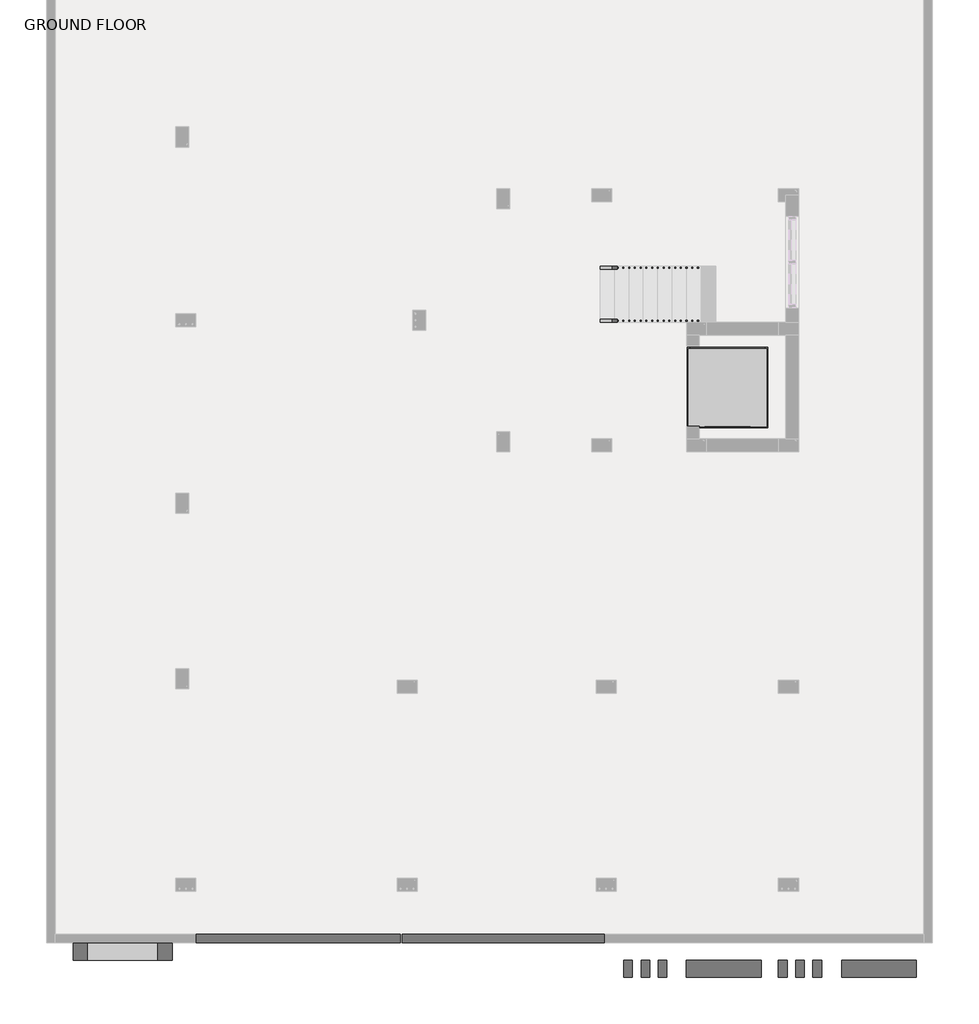
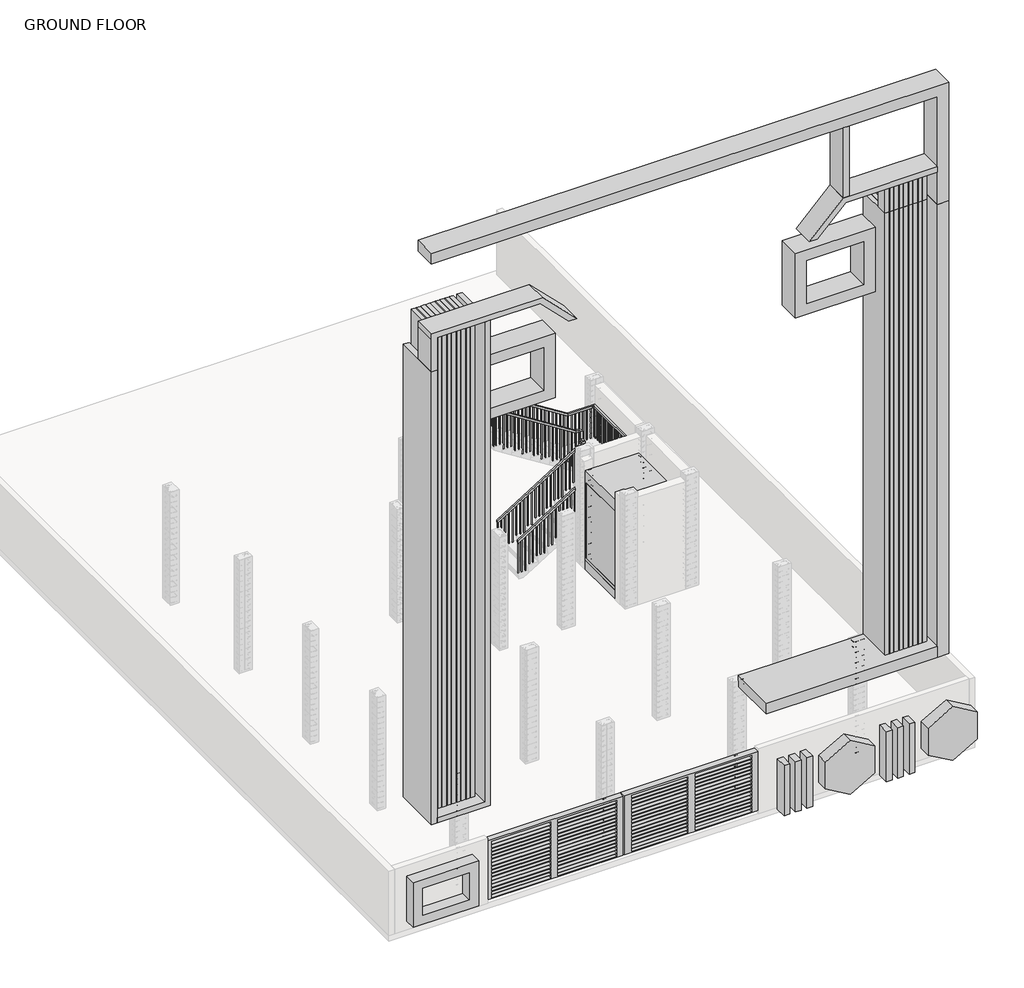
# One storey, part 2 of 7: 2 proxies, 2 railings.
"""IFC4 building model written with IfcOpenShell, lengths in millimetres."""

from ifc_helpers import new_model, si_unit, frame, origin, place, context, project, spatial, polyline, outline, extrude, faceted_brep, transform, mapped, element, save
from components import generic_models_4_generic_models_1_75103227, lift_glass_2_lift_with_hydraulic_ram_a28bd677

model = new_model("IFC4")

# Units and contexts
model_context = context("Model", 3, world=origin())
ifc_project = project(units=[si_unit("LENGTHUNIT", "METRE", prefix="MILLI")], contexts=[model_context])

# Site, building, storey
site = spatial("IfcSite", under=ifc_project)
building = spatial("IfcBuilding", under=site)
storey = spatial("IfcBuildingStorey", under=building, Name="GROUND FLOOR", Elevation=0.0)

# Proxies
placement = place(None, origin())
generic_models_4_generic_models_1_shape = generic_models_4_generic_models_1_75103227(model_context)
element("IfcBuildingElementProxy", 1, Name="Generic Models 4 : Generic Models 1", ObjectType="Generic Models 4 : Generic Models 1", at=placement, inside=storey, context=model_context, shape_type="MappedRepresentation", body=[
    mapped(generic_models_4_generic_models_1_shape, transform((0.0, 0.0, 0.0), x_axis=(1.0, 0.0, 0.0), y_axis=(0.0, 1.0, 0.0), z_axis=(0.0, 0.0, 1.0))),
])
lift_glass_2_lift_with_hydraulic_ram_shape = lift_glass_2_lift_with_hydraulic_ram_a28bd677(model_context)
element("IfcBuildingElementProxy", 2, Name="Lift Glass (2) : Lift with Hydraulic Ram", ObjectType="Lift Glass (2) : Lift with Hydraulic Ram", at=placement, inside=storey, context=model_context, shape_type="MappedRepresentation", body=[
    mapped(lift_glass_2_lift_with_hydraulic_ram_shape, transform((3468.4307677, -1196.2226692, 252.7510845), x_axis=(1.0, 0.0, 0.0), y_axis=(0.0, 1.0, 0.0), z_axis=(0.0, 0.0, 1.0))),
])

# Railings
element("IfcRailing", 3, ObjectType="Handrail - Rectangular", at=placement, inside=storey, context=model_context, shape_type="SolidModel", body=[
    faceted_brep([(1253.5166213, 60.259934, 1074.42), (1253.5166213, 60.259934, 1014.3792137), (1253.5166213, 9.459934, 1014.3792137), (1253.5166213, 9.459934, 1074.42), (3539.5166213, 60.259934, 2514.6), (3554.184536, 60.259934, 2463.8), (3554.184536, 9.459934, 2463.8), (3539.5166213, 9.459934, 2514.6), (4479.3166213, 60.259934, 2514.6), (4479.3166213, 60.259934, 2463.8), (4530.1166213, 9.459934, 2463.8), (4530.1166213, 9.459934, 2514.6), (4479.3166213, 2092.259934, 2514.6), (4479.3166213, 2092.259934, 2463.8), (4530.1166213, 2143.059934, 2463.8), (4530.1166213, 2143.059934, 2514.6), (3793.5166213, 2092.259934, 2514.6), (3778.8487066, 2092.259934, 2463.8), (3778.8487066, 2143.059934, 2463.8), (3793.5166213, 2143.059934, 2514.6), (1253.5166213, 2092.259934, 4114.8), (1253.5166213, 2143.059934, 4114.8), (1253.5166213, 2143.059934, 4054.7592137), (1253.5166213, 2092.259934, 4054.7592137)], [[[0, 1, 2, 3]], [[1, 0, 4, 5]], [[2, 1, 5, 6]], [[3, 2, 6, 7]], [[0, 3, 7, 4]], [[5, 4, 8, 9]], [[6, 5, 9, 10]], [[7, 6, 10, 11]], [[4, 7, 11, 8]], [[9, 8, 12, 13]], [[10, 9, 13, 14]], [[11, 10, 14, 15]], [[8, 11, 15, 12]], [[13, 12, 16, 17]], [[14, 13, 17, 18]], [[15, 14, 18, 19]], [[12, 15, 19, 16]], [[20, 21, 22, 23]], [[17, 16, 20, 23]], [[18, 17, 23, 22]], [[19, 18, 22, 21]], [[16, 19, 21, 20]]]),
    extrude(outline(polyline([(3984.7504637, 1364.6416213), (3996.7519637, 1345.5916213), (3040.38, 1345.5916213), (3040.38, 1364.6416213), (3984.7504637, 1364.6416213)])), frame((0.0, 2108.134934, 0.0), z_axis=(0.0, 1.0, 0.0), x_axis=(0.0, 0.0, 1.0)), (0.0, 0.0, 1.0), 19.05),
    extrude(outline(polyline([(3920.7424637, 1466.2416213), (3932.7439637, 1447.1916213), (3040.38, 1447.1916213), (3040.38, 1466.2416213), (3920.7424637, 1466.2416213)])), frame((0.0, 2108.134934, 0.0), z_axis=(0.0, 1.0, 0.0), x_axis=(0.0, 0.0, 1.0)), (0.0, 0.0, 1.0), 19.05),
    extrude(outline(polyline([(3856.7344637, 1567.8416213), (3868.7359637, 1548.7916213), (2880.36, 1548.7916213), (2880.36, 1567.8416213), (3856.7344637, 1567.8416213)])), frame((0.0, 2108.134934, 0.0), z_axis=(0.0, 1.0, 0.0), x_axis=(0.0, 0.0, 1.0)), (0.0, 0.0, 1.0), 19.05),
    extrude(outline(polyline([(3792.7264637, 1669.4416213), (3804.7279637, 1650.3916213), (2880.36, 1650.3916213), (2880.36, 1669.4416213), (3792.7264637, 1669.4416213)])), frame((0.0, 2108.134934, 0.0), z_axis=(0.0, 1.0, 0.0), x_axis=(0.0, 0.0, 1.0)), (0.0, 0.0, 1.0), 19.05),
    extrude(outline(polyline([(3728.7184637, 1771.0416213), (3740.7199637, 1751.9916213), (2880.36, 1751.9916213), (2880.36, 1771.0416213), (3728.7184637, 1771.0416213)])), frame((0.0, 2108.134934, 0.0), z_axis=(0.0, 1.0, 0.0), x_axis=(0.0, 0.0, 1.0)), (0.0, 0.0, 1.0), 19.05),
    extrude(outline(polyline([(3664.7104637, 1872.6416213), (3676.7119637, 1853.5916213), (2720.34, 1853.5916213), (2720.34, 1872.6416213), (3664.7104637, 1872.6416213)])), frame((0.0, 2108.134934, 0.0), z_axis=(0.0, 1.0, 0.0), x_axis=(0.0, 0.0, 1.0)), (0.0, 0.0, 1.0), 19.05),
    extrude(outline(polyline([(3600.7024637, 1974.2416213), (3612.7039637, 1955.1916213), (2720.34, 1955.1916213), (2720.34, 1974.2416213), (3600.7024637, 1974.2416213)])), frame((0.0, 2108.134934, 0.0), z_axis=(0.0, 1.0, 0.0), x_axis=(0.0, 0.0, 1.0)), (0.0, 0.0, 1.0), 19.05),
    extrude(outline(polyline([(3536.6944637, 2075.8416213), (3548.6959637, 2056.7916213), (2560.32, 2056.7916213), (2560.32, 2075.8416213), (3536.6944637, 2075.8416213)])), frame((0.0, 2108.134934, 0.0), z_axis=(0.0, 1.0, 0.0), x_axis=(0.0, 0.0, 1.0)), (0.0, 0.0, 1.0), 19.05),
    extrude(outline(polyline([(3472.6864637, 2177.4416213), (3484.6879637, 2158.3916213), (2560.32, 2158.3916213), (2560.32, 2177.4416213), (3472.6864637, 2177.4416213)])), frame((0.0, 2108.134934, 0.0), z_axis=(0.0, 1.0, 0.0), x_axis=(0.0, 0.0, 1.0)), (0.0, 0.0, 1.0), 19.05),
    extrude(outline(polyline([(3408.6784637, 2279.0416213), (3420.6799637, 2259.9916213), (2560.32, 2259.9916213), (2560.32, 2279.0416213), (3408.6784637, 2279.0416213)])), frame((0.0, 2108.134934, 0.0), z_axis=(0.0, 1.0, 0.0), x_axis=(0.0, 0.0, 1.0)), (0.0, 0.0, 1.0), 19.05),
    extrude(outline(polyline([(3344.6704637, 2380.6416213), (3356.6719637, 2361.5916213), (2400.3, 2361.5916213), (2400.3, 2380.6416213), (3344.6704637, 2380.6416213)])), frame((0.0, 2108.134934, 0.0), z_axis=(0.0, 1.0, 0.0), x_axis=(0.0, 0.0, 1.0)), (0.0, 0.0, 1.0), 19.05),
    extrude(outline(polyline([(3280.6624637, 2482.2416213), (3292.6639637, 2463.1916213), (2400.3, 2463.1916213), (2400.3, 2482.2416213), (3280.6624637, 2482.2416213)])), frame((0.0, 2108.134934, 0.0), z_axis=(0.0, 1.0, 0.0), x_axis=(0.0, 0.0, 1.0)), (0.0, 0.0, 1.0), 19.05),
    extrude(outline(polyline([(3216.6544637, 2583.8416213), (3228.6559637, 2564.7916213), (2240.28, 2564.7916213), (2240.28, 2583.8416213), (3216.6544637, 2583.8416213)])), frame((0.0, 2108.134934, 0.0), z_axis=(0.0, 1.0, 0.0), x_axis=(0.0, 0.0, 1.0)), (0.0, 0.0, 1.0), 19.05),
    extrude(outline(polyline([(3152.6464637, 2685.4416213), (3164.6479637, 2666.3916213), (2240.28, 2666.3916213), (2240.28, 2685.4416213), (3152.6464637, 2685.4416213)])), frame((0.0, 2108.134934, 0.0), z_axis=(0.0, 1.0, 0.0), x_axis=(0.0, 0.0, 1.0)), (0.0, 0.0, 1.0), 19.05),
    extrude(outline(polyline([(3088.6384637, 2787.0416213), (3100.6399637, 2767.9916213), (2240.28, 2767.9916213), (2240.28, 2787.0416213), (3088.6384637, 2787.0416213)])), frame((0.0, 2108.134934, 0.0), z_axis=(0.0, 1.0, 0.0), x_axis=(0.0, 0.0, 1.0)), (0.0, 0.0, 1.0), 19.05),
    extrude(outline(polyline([(3024.6304637, 2888.6416213), (3036.6319637, 2869.5916213), (2080.26, 2869.5916213), (2080.26, 2888.6416213), (3024.6304637, 2888.6416213)])), frame((0.0, 2108.134934, 0.0), z_axis=(0.0, 1.0, 0.0), x_axis=(0.0, 0.0, 1.0)), (0.0, 0.0, 1.0), 19.05),
    extrude(outline(polyline([(2960.6224637, 2990.2416213), (2972.6239637, 2971.1916213), (2080.26, 2971.1916213), (2080.26, 2990.2416213), (2960.6224637, 2990.2416213)])), frame((0.0, 2108.134934, 0.0), z_axis=(0.0, 1.0, 0.0), x_axis=(0.0, 0.0, 1.0)), (0.0, 0.0, 1.0), 19.05),
    extrude(outline(polyline([(2896.6144637, 3091.8416213), (2908.6159637, 3072.7916213), (1920.24, 3072.7916213), (1920.24, 3091.8416213), (2896.6144637, 3091.8416213)])), frame((0.0, 2108.134934, 0.0), z_axis=(0.0, 1.0, 0.0), x_axis=(0.0, 0.0, 1.0)), (0.0, 0.0, 1.0), 19.05),
    extrude(outline(polyline([(2832.6064637, 3193.4416213), (2844.6079637, 3174.3916213), (1920.24, 3174.3916213), (1920.24, 3193.4416213), (2832.6064637, 3193.4416213)])), frame((0.0, 2108.134934, 0.0), z_axis=(0.0, 1.0, 0.0), x_axis=(0.0, 0.0, 1.0)), (0.0, 0.0, 1.0), 19.05),
    extrude(outline(polyline([(2768.5984637, 3295.0416213), (2780.5999637, 3275.9916213), (1920.24, 3275.9916213), (1920.24, 3295.0416213), (2768.5984637, 3295.0416213)])), frame((0.0, 2108.134934, 0.0), z_axis=(0.0, 1.0, 0.0), x_axis=(0.0, 0.0, 1.0)), (0.0, 0.0, 1.0), 19.05),
    extrude(outline(polyline([(2704.5904637, 3396.6416213), (2716.5919637, 3377.5916213), (1760.22, 3377.5916213), (1760.22, 3396.6416213), (2704.5904637, 3396.6416213)])), frame((0.0, 2108.134934, 0.0), z_axis=(0.0, 1.0, 0.0), x_axis=(0.0, 0.0, 1.0)), (0.0, 0.0, 1.0), 19.05),
    extrude(outline(polyline([(2640.5824637, 3498.2416213), (2652.5839637, 3479.1916213), (1760.22, 3479.1916213), (1760.22, 3498.2416213), (2640.5824637, 3498.2416213)])), frame((0.0, 2108.134934, 0.0), z_axis=(0.0, 1.0, 0.0), x_axis=(0.0, 0.0, 1.0)), (0.0, 0.0, 1.0), 19.05),
    extrude(outline(polyline([(2576.5744637, 3599.8416213), (2588.5759637, 3580.7916213), (1600.2, 3580.7916213), (1600.2, 3599.8416213), (2576.5744637, 3599.8416213)])), frame((0.0, 2108.134934, 0.0), z_axis=(0.0, 1.0, 0.0), x_axis=(0.0, 0.0, 1.0)), (0.0, 0.0, 1.0), 19.05),
    extrude(outline(polyline([(2512.5664637, 3701.4416213), (2524.5679637, 3682.3916213), (1600.2, 3682.3916213), (1600.2, 3701.4416213), (2512.5664637, 3701.4416213)])), frame((0.0, 2108.134934, 0.0), z_axis=(0.0, 1.0, 0.0), x_axis=(0.0, 0.0, 1.0)), (0.0, 0.0, 1.0), 19.05),
    extrude(outline(polyline([(3803.0416213, 2127.184934), (3803.0416213, 2108.134934), (3783.9916213, 2108.134934), (3783.9916213, 2127.184934), (3803.0416213, 2127.184934)])), frame((0.0, 0.0, 1600.2), z_axis=(0.0, 0.0, 1.0), x_axis=(1.0, 0.0, 0.0)), (0.0, 0.0, 1.0), 863.6),
    extrude(outline(polyline([(3904.6416213, 2127.184934), (3904.6416213, 2108.134934), (3885.5916213, 2108.134934), (3885.5916213, 2127.184934), (3904.6416213, 2127.184934)])), frame((0.0, 0.0, 1600.2), z_axis=(0.0, 0.0, 1.0), x_axis=(1.0, 0.0, 0.0)), (0.0, 0.0, 1.0), 863.6),
    extrude(outline(polyline([(4006.2416213, 2127.184934), (4006.2416213, 2108.134934), (3987.1916213, 2108.134934), (3987.1916213, 2127.184934), (4006.2416213, 2127.184934)])), frame((0.0, 0.0, 1600.2), z_axis=(0.0, 0.0, 1.0), x_axis=(1.0, 0.0, 0.0)), (0.0, 0.0, 1.0), 863.6),
    extrude(outline(polyline([(4107.8416213, 2127.184934), (4107.8416213, 2108.134934), (4088.7916213, 2108.134934), (4088.7916213, 2127.184934), (4107.8416213, 2127.184934)])), frame((0.0, 0.0, 1600.2), z_axis=(0.0, 0.0, 1.0), x_axis=(1.0, 0.0, 0.0)), (0.0, 0.0, 1.0), 863.6),
    extrude(outline(polyline([(4209.4416213, 2127.184934), (4209.4416213, 2108.134934), (4190.3916213, 2108.134934), (4190.3916213, 2127.184934), (4209.4416213, 2127.184934)])), frame((0.0, 0.0, 1600.2), z_axis=(0.0, 0.0, 1.0), x_axis=(1.0, 0.0, 0.0)), (0.0, 0.0, 1.0), 863.6),
    extrude(outline(polyline([(4311.0416213, 2127.184934), (4311.0416213, 2108.134934), (4291.9916213, 2108.134934), (4291.9916213, 2127.184934), (4311.0416213, 2127.184934)])), frame((0.0, 0.0, 1600.2), z_axis=(0.0, 0.0, 1.0), x_axis=(1.0, 0.0, 0.0)), (0.0, 0.0, 1.0), 863.6),
    extrude(outline(polyline([(4412.6416213, 2127.184934), (4412.6416213, 2108.134934), (4393.5916213, 2108.134934), (4393.5916213, 2127.184934), (4412.6416213, 2127.184934)])), frame((0.0, 0.0, 1600.2), z_axis=(0.0, 0.0, 1.0), x_axis=(1.0, 0.0, 0.0)), (0.0, 0.0, 1.0), 863.6),
    extrude(outline(polyline([(4514.2416213, 2057.334934), (4495.1916213, 2057.334934), (4495.1916213, 2076.384934), (4514.2416213, 2076.384934), (4514.2416213, 2057.334934)])), frame((0.0, 0.0, 1600.2), z_axis=(0.0, 0.0, 1.0), x_axis=(1.0, 0.0, 0.0)), (0.0, 0.0, 1.0), 863.6),
    extrude(outline(polyline([(4514.2416213, 1955.734934), (4495.1916213, 1955.734934), (4495.1916213, 1974.784934), (4514.2416213, 1974.784934), (4514.2416213, 1955.734934)])), frame((0.0, 0.0, 1600.2), z_axis=(0.0, 0.0, 1.0), x_axis=(1.0, 0.0, 0.0)), (0.0, 0.0, 1.0), 863.6),
    extrude(outline(polyline([(4514.2416213, 1854.134934), (4495.1916213, 1854.134934), (4495.1916213, 1873.184934), (4514.2416213, 1873.184934), (4514.2416213, 1854.134934)])), frame((0.0, 0.0, 1600.2), z_axis=(0.0, 0.0, 1.0), x_axis=(1.0, 0.0, 0.0)), (0.0, 0.0, 1.0), 863.6),
    extrude(outline(polyline([(4514.2416213, 1752.534934), (4495.1916213, 1752.534934), (4495.1916213, 1771.584934), (4514.2416213, 1771.584934), (4514.2416213, 1752.534934)])), frame((0.0, 0.0, 1600.2), z_axis=(0.0, 0.0, 1.0), x_axis=(1.0, 0.0, 0.0)), (0.0, 0.0, 1.0), 863.6),
    extrude(outline(polyline([(4514.2416213, 1650.934934), (4495.1916213, 1650.934934), (4495.1916213, 1669.984934), (4514.2416213, 1669.984934), (4514.2416213, 1650.934934)])), frame((0.0, 0.0, 1600.2), z_axis=(0.0, 0.0, 1.0), x_axis=(1.0, 0.0, 0.0)), (0.0, 0.0, 1.0), 863.6),
    extrude(outline(polyline([(4514.2416213, 1549.334934), (4495.1916213, 1549.334934), (4495.1916213, 1568.384934), (4514.2416213, 1568.384934), (4514.2416213, 1549.334934)])), frame((0.0, 0.0, 1600.2), z_axis=(0.0, 0.0, 1.0), x_axis=(1.0, 0.0, 0.0)), (0.0, 0.0, 1.0), 863.6),
    extrude(outline(polyline([(4514.2416213, 1447.734934), (4495.1916213, 1447.734934), (4495.1916213, 1466.784934), (4514.2416213, 1466.784934), (4514.2416213, 1447.734934)])), frame((0.0, 0.0, 1600.2), z_axis=(0.0, 0.0, 1.0), x_axis=(1.0, 0.0, 0.0)), (0.0, 0.0, 1.0), 863.6),
    extrude(outline(polyline([(4514.2416213, 1346.134934), (4495.1916213, 1346.134934), (4495.1916213, 1365.184934), (4514.2416213, 1365.184934), (4514.2416213, 1346.134934)])), frame((0.0, 0.0, 1600.2), z_axis=(0.0, 0.0, 1.0), x_axis=(1.0, 0.0, 0.0)), (0.0, 0.0, 1.0), 863.6),
    extrude(outline(polyline([(4514.2416213, 1244.534934), (4495.1916213, 1244.534934), (4495.1916213, 1263.584934), (4514.2416213, 1263.584934), (4514.2416213, 1244.534934)])), frame((0.0, 0.0, 1600.2), z_axis=(0.0, 0.0, 1.0), x_axis=(1.0, 0.0, 0.0)), (0.0, 0.0, 1.0), 863.6),
    extrude(outline(polyline([(4514.2416213, 1142.934934), (4495.1916213, 1142.934934), (4495.1916213, 1161.984934), (4514.2416213, 1161.984934), (4514.2416213, 1142.934934)])), frame((0.0, 0.0, 1600.2), z_axis=(0.0, 0.0, 1.0), x_axis=(1.0, 0.0, 0.0)), (0.0, 0.0, 1.0), 863.6),
    extrude(outline(polyline([(4514.2416213, 1041.334934), (4495.1916213, 1041.334934), (4495.1916213, 1060.384934), (4514.2416213, 1060.384934), (4514.2416213, 1041.334934)])), frame((0.0, 0.0, 1600.2), z_axis=(0.0, 0.0, 1.0), x_axis=(1.0, 0.0, 0.0)), (0.0, 0.0, 1.0), 863.6),
    extrude(outline(polyline([(4514.2416213, 939.734934), (4495.1916213, 939.734934), (4495.1916213, 958.784934), (4514.2416213, 958.784934), (4514.2416213, 939.734934)])), frame((0.0, 0.0, 1600.2), z_axis=(0.0, 0.0, 1.0), x_axis=(1.0, 0.0, 0.0)), (0.0, 0.0, 1.0), 863.6),
    extrude(outline(polyline([(4514.2416213, 838.134934), (4495.1916213, 838.134934), (4495.1916213, 857.184934), (4514.2416213, 857.184934), (4514.2416213, 838.134934)])), frame((0.0, 0.0, 1600.2), z_axis=(0.0, 0.0, 1.0), x_axis=(1.0, 0.0, 0.0)), (0.0, 0.0, 1.0), 863.6),
    extrude(outline(polyline([(4514.2416213, 736.534934), (4495.1916213, 736.534934), (4495.1916213, 755.584934), (4514.2416213, 755.584934), (4514.2416213, 736.534934)])), frame((0.0, 0.0, 1600.2), z_axis=(0.0, 0.0, 1.0), x_axis=(1.0, 0.0, 0.0)), (0.0, 0.0, 1.0), 863.6),
    extrude(outline(polyline([(4514.2416213, 634.934934), (4495.1916213, 634.934934), (4495.1916213, 653.984934), (4514.2416213, 653.984934), (4514.2416213, 634.934934)])), frame((0.0, 0.0, 1600.2), z_axis=(0.0, 0.0, 1.0), x_axis=(1.0, 0.0, 0.0)), (0.0, 0.0, 1.0), 863.6),
    extrude(outline(polyline([(4514.2416213, 533.334934), (4495.1916213, 533.334934), (4495.1916213, 552.384934), (4514.2416213, 552.384934), (4514.2416213, 533.334934)])), frame((0.0, 0.0, 1600.2), z_axis=(0.0, 0.0, 1.0), x_axis=(1.0, 0.0, 0.0)), (0.0, 0.0, 1.0), 863.6),
    extrude(outline(polyline([(4514.2416213, 431.734934), (4495.1916213, 431.734934), (4495.1916213, 450.784934), (4514.2416213, 450.784934), (4514.2416213, 431.734934)])), frame((0.0, 0.0, 1600.2), z_axis=(0.0, 0.0, 1.0), x_axis=(1.0, 0.0, 0.0)), (0.0, 0.0, 1.0), 863.6),
    extrude(outline(polyline([(4514.2416213, 330.134934), (4495.1916213, 330.134934), (4495.1916213, 349.184934), (4514.2416213, 349.184934), (4514.2416213, 330.134934)])), frame((0.0, 0.0, 1600.2), z_axis=(0.0, 0.0, 1.0), x_axis=(1.0, 0.0, 0.0)), (0.0, 0.0, 1.0), 863.6),
    extrude(outline(polyline([(4514.2416213, 228.534934), (4495.1916213, 228.534934), (4495.1916213, 247.584934), (4514.2416213, 247.584934), (4514.2416213, 228.534934)])), frame((0.0, 0.0, 1600.2), z_axis=(0.0, 0.0, 1.0), x_axis=(1.0, 0.0, 0.0)), (0.0, 0.0, 1.0), 863.6),
    extrude(outline(polyline([(4514.2416213, 126.934934), (4495.1916213, 126.934934), (4495.1916213, 145.984934), (4514.2416213, 145.984934), (4514.2416213, 126.934934)])), frame((0.0, 0.0, 1600.2), z_axis=(0.0, 0.0, 1.0), x_axis=(1.0, 0.0, 0.0)), (0.0, 0.0, 1.0), 863.6),
    extrude(outline(polyline([(4393.5916213, 25.334934), (4393.5916213, 44.384934), (4412.6416213, 44.384934), (4412.6416213, 25.334934), (4393.5916213, 25.334934)])), frame((0.0, 0.0, 1600.2), z_axis=(0.0, 0.0, 1.0), x_axis=(1.0, 0.0, 0.0)), (0.0, 0.0, 1.0), 863.6),
    extrude(outline(polyline([(4291.9916213, 25.334934), (4291.9916213, 44.384934), (4311.0416213, 44.384934), (4311.0416213, 25.334934), (4291.9916213, 25.334934)])), frame((0.0, 0.0, 1600.2), z_axis=(0.0, 0.0, 1.0), x_axis=(1.0, 0.0, 0.0)), (0.0, 0.0, 1.0), 863.6),
    extrude(outline(polyline([(4190.3916213, 25.334934), (4190.3916213, 44.384934), (4209.4416213, 44.384934), (4209.4416213, 25.334934), (4190.3916213, 25.334934)])), frame((0.0, 0.0, 1600.2), z_axis=(0.0, 0.0, 1.0), x_axis=(1.0, 0.0, 0.0)), (0.0, 0.0, 1.0), 863.6),
    extrude(outline(polyline([(4088.7916213, 25.334934), (4088.7916213, 44.384934), (4107.8416213, 44.384934), (4107.8416213, 25.334934), (4088.7916213, 25.334934)])), frame((0.0, 0.0, 1600.2), z_axis=(0.0, 0.0, 1.0), x_axis=(1.0, 0.0, 0.0)), (0.0, 0.0, 1.0), 863.6),
    extrude(outline(polyline([(3987.1916213, 25.334934), (3987.1916213, 44.384934), (4006.2416213, 44.384934), (4006.2416213, 25.334934), (3987.1916213, 25.334934)])), frame((0.0, 0.0, 1600.2), z_axis=(0.0, 0.0, 1.0), x_axis=(1.0, 0.0, 0.0)), (0.0, 0.0, 1.0), 863.6),
    extrude(outline(polyline([(3885.5916213, 25.334934), (3885.5916213, 44.384934), (3904.6416213, 44.384934), (3904.6416213, 25.334934), (3885.5916213, 25.334934)])), frame((0.0, 0.0, 1600.2), z_axis=(0.0, 0.0, 1.0), x_axis=(1.0, 0.0, 0.0)), (0.0, 0.0, 1.0), 863.6),
    extrude(outline(polyline([(3783.9916213, 25.334934), (3783.9916213, 44.384934), (3803.0416213, 44.384934), (3803.0416213, 25.334934), (3783.9916213, 25.334934)])), frame((0.0, 0.0, 1600.2), z_axis=(0.0, 0.0, 1.0), x_axis=(1.0, 0.0, 0.0)), (0.0, 0.0, 1.0), 863.6),
    extrude(outline(polyline([(3682.3916213, 25.334934), (3682.3916213, 44.384934), (3701.4416213, 44.384934), (3701.4416213, 25.334934), (3682.3916213, 25.334934)])), frame((0.0, 0.0, 1600.2), z_axis=(0.0, 0.0, 1.0), x_axis=(1.0, 0.0, 0.0)), (0.0, 0.0, 1.0), 863.6),
    extrude(outline(polyline([(3580.7916213, 25.334934), (3580.7916213, 44.384934), (3599.8416213, 44.384934), (3599.8416213, 25.334934), (3580.7916213, 25.334934)])), frame((0.0, 0.0, 1600.2), z_axis=(0.0, 0.0, 1.0), x_axis=(1.0, 0.0, 0.0)), (0.0, 0.0, 1.0), 863.6),
    extrude(outline(polyline([(2428.5559637, 3498.2416213), (2416.5544637, 3479.1916213), (1440.18, 3479.1916213), (1440.18, 3498.2416213), (2428.5559637, 3498.2416213)])), frame((0.0, 25.334934, 0.0), z_axis=(0.0, 1.0, 0.0), x_axis=(0.0, 0.0, 1.0)), (0.0, 0.0, 1.0), 19.05),
    extrude(outline(polyline([(2364.5479637, 3396.6416213), (2352.5464637, 3377.5916213), (1440.18, 3377.5916213), (1440.18, 3396.6416213), (2364.5479637, 3396.6416213)])), frame((0.0, 25.334934, 0.0), z_axis=(0.0, 1.0, 0.0), x_axis=(0.0, 0.0, 1.0)), (0.0, 0.0, 1.0), 19.05),
    extrude(outline(polyline([(2300.5399637, 3295.0416213), (2288.5384637, 3275.9916213), (1440.18, 3275.9916213), (1440.18, 3295.0416213), (2300.5399637, 3295.0416213)])), frame((0.0, 25.334934, 0.0), z_axis=(0.0, 1.0, 0.0), x_axis=(0.0, 0.0, 1.0)), (0.0, 0.0, 1.0), 19.05),
    extrude(outline(polyline([(2236.5319637, 3193.4416213), (2224.5304637, 3174.3916213), (1280.16, 3174.3916213), (1280.16, 3193.4416213), (2236.5319637, 3193.4416213)])), frame((0.0, 25.334934, 0.0), z_axis=(0.0, 1.0, 0.0), x_axis=(0.0, 0.0, 1.0)), (0.0, 0.0, 1.0), 19.05),
    extrude(outline(polyline([(2172.5239637, 3091.8416213), (2160.5224637, 3072.7916213), (1280.16, 3072.7916213), (1280.16, 3091.8416213), (2172.5239637, 3091.8416213)])), frame((0.0, 25.334934, 0.0), z_axis=(0.0, 1.0, 0.0), x_axis=(0.0, 0.0, 1.0)), (0.0, 0.0, 1.0), 19.05),
    extrude(outline(polyline([(2108.5159637, 2990.2416213), (2096.5144637, 2971.1916213), (1120.14, 2971.1916213), (1120.14, 2990.2416213), (2108.5159637, 2990.2416213)])), frame((0.0, 25.334934, 0.0), z_axis=(0.0, 1.0, 0.0), x_axis=(0.0, 0.0, 1.0)), (0.0, 0.0, 1.0), 19.05),
    extrude(outline(polyline([(2044.5079637, 2888.6416213), (2032.5064637, 2869.5916213), (1120.14, 2869.5916213), (1120.14, 2888.6416213), (2044.5079637, 2888.6416213)])), frame((0.0, 25.334934, 0.0), z_axis=(0.0, 1.0, 0.0), x_axis=(0.0, 0.0, 1.0)), (0.0, 0.0, 1.0), 19.05),
    extrude(outline(polyline([(1980.4999637, 2787.0416213), (1968.4984637, 2767.9916213), (1120.14, 2767.9916213), (1120.14, 2787.0416213), (1980.4999637, 2787.0416213)])), frame((0.0, 25.334934, 0.0), z_axis=(0.0, 1.0, 0.0), x_axis=(0.0, 0.0, 1.0)), (0.0, 0.0, 1.0), 19.05),
    extrude(outline(polyline([(1916.4919637, 2685.4416213), (1904.4904637, 2666.3916213), (960.12, 2666.3916213), (960.12, 2685.4416213), (1916.4919637, 2685.4416213)])), frame((0.0, 25.334934, 0.0), z_axis=(0.0, 1.0, 0.0), x_axis=(0.0, 0.0, 1.0)), (0.0, 0.0, 1.0), 19.05),
    extrude(outline(polyline([(1852.4839637, 2583.8416213), (1840.4824637, 2564.7916213), (960.12, 2564.7916213), (960.12, 2583.8416213), (1852.4839637, 2583.8416213)])), frame((0.0, 25.334934, 0.0), z_axis=(0.0, 1.0, 0.0), x_axis=(0.0, 0.0, 1.0)), (0.0, 0.0, 1.0), 19.05),
    extrude(outline(polyline([(1788.4759637, 2482.2416213), (1776.4744637, 2463.1916213), (800.1, 2463.1916213), (800.1, 2482.2416213), (1788.4759637, 2482.2416213)])), frame((0.0, 25.334934, 0.0), z_axis=(0.0, 1.0, 0.0), x_axis=(0.0, 0.0, 1.0)), (0.0, 0.0, 1.0), 19.05),
    extrude(outline(polyline([(1724.4679637, 2380.6416213), (1712.4664637, 2361.5916213), (800.1, 2361.5916213), (800.1, 2380.6416213), (1724.4679637, 2380.6416213)])), frame((0.0, 25.334934, 0.0), z_axis=(0.0, 1.0, 0.0), x_axis=(0.0, 0.0, 1.0)), (0.0, 0.0, 1.0), 19.05),
    extrude(outline(polyline([(1660.4599637, 2279.0416213), (1648.4584637, 2259.9916213), (800.1, 2259.9916213), (800.1, 2279.0416213), (1660.4599637, 2279.0416213)])), frame((0.0, 25.334934, 0.0), z_axis=(0.0, 1.0, 0.0), x_axis=(0.0, 0.0, 1.0)), (0.0, 0.0, 1.0), 19.05),
    extrude(outline(polyline([(1596.4519637, 2177.4416213), (1584.4504637, 2158.3916213), (640.08, 2158.3916213), (640.08, 2177.4416213), (1596.4519637, 2177.4416213)])), frame((0.0, 25.334934, 0.0), z_axis=(0.0, 1.0, 0.0), x_axis=(0.0, 0.0, 1.0)), (0.0, 0.0, 1.0), 19.05),
    extrude(outline(polyline([(1532.4439637, 2075.8416213), (1520.4424637, 2056.7916213), (640.08, 2056.7916213), (640.08, 2075.8416213), (1532.4439637, 2075.8416213)])), frame((0.0, 25.334934, 0.0), z_axis=(0.0, 1.0, 0.0), x_axis=(0.0, 0.0, 1.0)), (0.0, 0.0, 1.0), 19.05),
    extrude(outline(polyline([(1468.4359637, 1974.2416213), (1456.4344637, 1955.1916213), (480.06, 1955.1916213), (480.06, 1974.2416213), (1468.4359637, 1974.2416213)])), frame((0.0, 25.334934, 0.0), z_axis=(0.0, 1.0, 0.0), x_axis=(0.0, 0.0, 1.0)), (0.0, 0.0, 1.0), 19.05),
    extrude(outline(polyline([(1404.4279637, 1872.6416213), (1392.4264637, 1853.5916213), (480.06, 1853.5916213), (480.06, 1872.6416213), (1404.4279637, 1872.6416213)])), frame((0.0, 25.334934, 0.0), z_axis=(0.0, 1.0, 0.0), x_axis=(0.0, 0.0, 1.0)), (0.0, 0.0, 1.0), 19.05),
    extrude(outline(polyline([(1340.4199637, 1771.0416213), (1328.4184637, 1751.9916213), (480.06, 1751.9916213), (480.06, 1771.0416213), (1340.4199637, 1771.0416213)])), frame((0.0, 25.334934, 0.0), z_axis=(0.0, 1.0, 0.0), x_axis=(0.0, 0.0, 1.0)), (0.0, 0.0, 1.0), 19.05),
    extrude(outline(polyline([(1276.4119637, 1669.4416213), (1264.4104637, 1650.3916213), (320.04, 1650.3916213), (320.04, 1669.4416213), (1276.4119637, 1669.4416213)])), frame((0.0, 25.334934, 0.0), z_axis=(0.0, 1.0, 0.0), x_axis=(0.0, 0.0, 1.0)), (0.0, 0.0, 1.0), 19.05),
    extrude(outline(polyline([(1212.4039637, 1567.8416213), (1200.4024637, 1548.7916213), (320.04, 1548.7916213), (320.04, 1567.8416213), (1212.4039637, 1567.8416213)])), frame((0.0, 25.334934, 0.0), z_axis=(0.0, 1.0, 0.0), x_axis=(0.0, 0.0, 1.0)), (0.0, 0.0, 1.0), 19.05),
    extrude(outline(polyline([(1148.3959637, 1466.2416213), (1136.3944637, 1447.1916213), (160.02, 1447.1916213), (160.02, 1466.2416213), (1148.3959637, 1466.2416213)])), frame((0.0, 25.334934, 0.0), z_axis=(0.0, 1.0, 0.0), x_axis=(0.0, 0.0, 1.0)), (0.0, 0.0, 1.0), 19.05),
    extrude(outline(polyline([(1084.3879637, 1364.6416213), (1072.3864637, 1345.5916213), (160.02, 1345.5916213), (160.02, 1364.6416213), (1084.3879637, 1364.6416213)])), frame((0.0, 25.334934, 0.0), z_axis=(0.0, 1.0, 0.0), x_axis=(0.0, 0.0, 1.0)), (0.0, 0.0, 1.0), 19.05),
    extrude(outline(polyline([(4514.2416213, 2108.134934), (4495.1916213, 2108.134934), (4495.1916213, 2127.184934), (4514.2416213, 2127.184934), (4514.2416213, 2108.134934)])), frame((0.0, 0.0, 1600.2), z_axis=(0.0, 0.0, 1.0), x_axis=(1.0, 0.0, 0.0)), (0.0, 0.0, 1.0), 863.6),
    extrude(outline(polyline([(4495.1916213, 25.334934), (4495.1916213, 44.384934), (4514.2416213, 44.384934), (4514.2416213, 25.334934), (4495.1916213, 25.334934)])), frame((0.0, 0.0, 1600.2), z_axis=(0.0, 0.0, 1.0), x_axis=(1.0, 0.0, 0.0)), (0.0, 0.0, 1.0), 863.6),
    extrude(outline(polyline([(4042.7577137, 1272.5666213), (4054.7592137, 1253.5166213), (3040.38, 1253.5166213), (3040.38, 1272.5666213), (4042.7577137, 1272.5666213)])), frame((0.0, 2108.134934, 0.0), z_axis=(0.0, 1.0, 0.0), x_axis=(0.0, 0.0, 1.0)), (0.0, 0.0, 1.0), 19.05),
    extrude(outline(polyline([(1026.3807137, 1272.5666213), (1014.3792137, 1253.5166213), (160.02, 1253.5166213), (160.02, 1272.5666213), (1026.3807137, 1272.5666213)])), frame((0.0, 25.334934, 0.0), z_axis=(0.0, 1.0, 0.0), x_axis=(0.0, 0.0, 1.0)), (0.0, 0.0, 1.0), 19.05),
])
element("IfcRailing", 4, ObjectType="Handrail - Rectangular", at=placement, inside=storey, context=model_context, shape_type="SolidModel", body=[
    faceted_brep([(1253.5166213, 1000.059934, 1074.42), (1253.5166213, 1000.059934, 1014.3792137), (1253.5166213, 949.259934, 1014.3792137), (1253.5166213, 949.259934, 1074.42), (3463.3166213, 1000.059934, 2466.594), (3514.1166213, 1000.059934, 2438.5572137), (3514.1166213, 949.259934, 2438.5572137), (3463.3166213, 949.259934, 2466.594), (3463.3166213, 1000.059934, 2514.6), (3514.1166213, 1000.059934, 2463.8), (3514.1166213, 949.259934, 2463.8), (3463.3166213, 949.259934, 2514.6), (3539.5166213, 1000.059934, 2514.6), (3539.5166213, 1000.059934, 2463.8), (3590.3166213, 949.259934, 2463.8), (3590.3166213, 949.259934, 2514.6), (3539.5166213, 1076.259934, 2514.6), (3539.5166213, 1127.059934, 2463.8), (3590.3166213, 1127.059934, 2463.8), (3590.3166213, 1076.259934, 2514.6), (3539.5166213, 1076.259934, 2722.626), (3539.5166213, 1127.059934, 2671.826), (3590.3166213, 1127.059934, 2671.826), (3590.3166213, 1076.259934, 2722.626), (3539.5166213, 1152.459934, 2722.626), (3539.5166213, 1152.459934, 2671.826), (3590.3166213, 1203.259934, 2671.826), (3590.3166213, 1203.259934, 2722.626), (3463.3166213, 1152.459934, 2722.626), (3448.6487066, 1152.459934, 2671.826), (3448.6487066, 1203.259934, 2671.826), (3463.3166213, 1203.259934, 2722.626), (1253.5166213, 1152.459934, 4114.8), (1253.5166213, 1203.259934, 4114.8), (1253.5166213, 1203.259934, 4054.7592137), (1253.5166213, 1152.459934, 4054.7592137)], [[[0, 1, 2, 3]], [[1, 0, 4, 5]], [[2, 1, 5, 6]], [[3, 2, 6, 7]], [[0, 3, 7, 4]], [[5, 4, 8, 9]], [[6, 5, 9, 10]], [[7, 6, 10, 11]], [[4, 7, 11, 8]], [[9, 8, 12, 13]], [[10, 9, 13, 14]], [[11, 10, 14, 15]], [[8, 11, 15, 12]], [[13, 12, 16, 17]], [[14, 13, 17, 18]], [[15, 14, 18, 19]], [[12, 15, 19, 16]], [[17, 16, 20, 21]], [[18, 17, 21, 22]], [[19, 18, 22, 23]], [[16, 19, 23, 20]], [[21, 20, 24, 25]], [[22, 21, 25, 26]], [[23, 22, 26, 27]], [[20, 23, 27, 24]], [[25, 24, 28, 29]], [[26, 25, 29, 30]], [[27, 26, 30, 31]], [[24, 27, 31, 28]], [[32, 33, 34, 35]], [[29, 28, 32, 35]], [[30, 29, 35, 34]], [[31, 30, 34, 33]], [[28, 31, 33, 32]]]),
    extrude(outline(polyline([(4012.7539637, 1320.1916213), (3040.38, 1320.1916213), (3040.38, 1339.2416213), (4000.7524637, 1339.2416213), (4012.7539637, 1320.1916213)])), frame((0.0, 1168.334934, 0.0), z_axis=(0.0, 1.0, 0.0), x_axis=(0.0, 0.0, 1.0)), (0.0, 0.0, 1.0), 19.05),
    extrude(outline(polyline([(3948.7459637, 1421.7916213), (3040.38, 1421.7916213), (3040.38, 1440.8416213), (3936.7444637, 1440.8416213), (3948.7459637, 1421.7916213)])), frame((0.0, 1168.334934, 0.0), z_axis=(0.0, 1.0, 0.0), x_axis=(0.0, 0.0, 1.0)), (0.0, 0.0, 1.0), 19.05),
    extrude(outline(polyline([(3884.7379637, 1523.3916213), (2880.36, 1523.3916213), (2880.36, 1542.4416213), (3872.7364637, 1542.4416213), (3884.7379637, 1523.3916213)])), frame((0.0, 1168.334934, 0.0), z_axis=(0.0, 1.0, 0.0), x_axis=(0.0, 0.0, 1.0)), (0.0, 0.0, 1.0), 19.05),
    extrude(outline(polyline([(3820.7299637, 1624.9916213), (2880.36, 1624.9916213), (2880.36, 1644.0416213), (3808.7284637, 1644.0416213), (3820.7299637, 1624.9916213)])), frame((0.0, 1168.334934, 0.0), z_axis=(0.0, 1.0, 0.0), x_axis=(0.0, 0.0, 1.0)), (0.0, 0.0, 1.0), 19.05),
    extrude(outline(polyline([(3756.7219637, 1726.5916213), (2880.36, 1726.5916213), (2880.36, 1745.6416213), (3744.7204637, 1745.6416213), (3756.7219637, 1726.5916213)])), frame((0.0, 1168.334934, 0.0), z_axis=(0.0, 1.0, 0.0), x_axis=(0.0, 0.0, 1.0)), (0.0, 0.0, 1.0), 19.05),
    extrude(outline(polyline([(3692.7139637, 1828.1916213), (2720.34, 1828.1916213), (2720.34, 1847.2416213), (3680.7124637, 1847.2416213), (3692.7139637, 1828.1916213)])), frame((0.0, 1168.334934, 0.0), z_axis=(0.0, 1.0, 0.0), x_axis=(0.0, 0.0, 1.0)), (0.0, 0.0, 1.0), 19.05),
    extrude(outline(polyline([(3628.7059637, 1929.7916213), (2720.34, 1929.7916213), (2720.34, 1948.8416213), (3616.7044637, 1948.8416213), (3628.7059637, 1929.7916213)])), frame((0.0, 1168.334934, 0.0), z_axis=(0.0, 1.0, 0.0), x_axis=(0.0, 0.0, 1.0)), (0.0, 0.0, 1.0), 19.05),
    extrude(outline(polyline([(3564.6979637, 2031.3916213), (2560.32, 2031.3916213), (2560.32, 2050.4416213), (3552.6964637, 2050.4416213), (3564.6979637, 2031.3916213)])), frame((0.0, 1168.334934, 0.0), z_axis=(0.0, 1.0, 0.0), x_axis=(0.0, 0.0, 1.0)), (0.0, 0.0, 1.0), 19.05),
    extrude(outline(polyline([(3500.6899637, 2132.9916213), (2560.32, 2132.9916213), (2560.32, 2152.0416213), (3488.6884637, 2152.0416213), (3500.6899637, 2132.9916213)])), frame((0.0, 1168.334934, 0.0), z_axis=(0.0, 1.0, 0.0), x_axis=(0.0, 0.0, 1.0)), (0.0, 0.0, 1.0), 19.05),
    extrude(outline(polyline([(3436.6819637, 2234.5916213), (2560.32, 2234.5916213), (2560.32, 2253.6416213), (3424.6804637, 2253.6416213), (3436.6819637, 2234.5916213)])), frame((0.0, 1168.334934, 0.0), z_axis=(0.0, 1.0, 0.0), x_axis=(0.0, 0.0, 1.0)), (0.0, 0.0, 1.0), 19.05),
    extrude(outline(polyline([(3372.6739637, 2336.1916213), (2400.3, 2336.1916213), (2400.3, 2355.2416213), (3360.6724637, 2355.2416213), (3372.6739637, 2336.1916213)])), frame((0.0, 1168.334934, 0.0), z_axis=(0.0, 1.0, 0.0), x_axis=(0.0, 0.0, 1.0)), (0.0, 0.0, 1.0), 19.05),
    extrude(outline(polyline([(3308.6659637, 2437.7916213), (2400.3, 2437.7916213), (2400.3, 2456.8416213), (3296.6644637, 2456.8416213), (3308.6659637, 2437.7916213)])), frame((0.0, 1168.334934, 0.0), z_axis=(0.0, 1.0, 0.0), x_axis=(0.0, 0.0, 1.0)), (0.0, 0.0, 1.0), 19.05),
    extrude(outline(polyline([(3244.6579637, 2539.3916213), (2240.28, 2539.3916213), (2240.28, 2558.4416213), (3232.6564637, 2558.4416213), (3244.6579637, 2539.3916213)])), frame((0.0, 1168.334934, 0.0), z_axis=(0.0, 1.0, 0.0), x_axis=(0.0, 0.0, 1.0)), (0.0, 0.0, 1.0), 19.05),
    extrude(outline(polyline([(3180.6499637, 2640.9916213), (2240.28, 2640.9916213), (2240.28, 2660.0416213), (3168.6484637, 2660.0416213), (3180.6499637, 2640.9916213)])), frame((0.0, 1168.334934, 0.0), z_axis=(0.0, 1.0, 0.0), x_axis=(0.0, 0.0, 1.0)), (0.0, 0.0, 1.0), 19.05),
    extrude(outline(polyline([(3116.6419637, 2742.5916213), (2240.28, 2742.5916213), (2240.28, 2761.6416213), (3104.6404637, 2761.6416213), (3116.6419637, 2742.5916213)])), frame((0.0, 1168.334934, 0.0), z_axis=(0.0, 1.0, 0.0), x_axis=(0.0, 0.0, 1.0)), (0.0, 0.0, 1.0), 19.05),
    extrude(outline(polyline([(3052.6339637, 2844.1916213), (2080.26, 2844.1916213), (2080.26, 2863.2416213), (3040.6324637, 2863.2416213), (3052.6339637, 2844.1916213)])), frame((0.0, 1168.334934, 0.0), z_axis=(0.0, 1.0, 0.0), x_axis=(0.0, 0.0, 1.0)), (0.0, 0.0, 1.0), 19.05),
    extrude(outline(polyline([(2988.6259637, 2945.7916213), (2080.26, 2945.7916213), (2080.26, 2964.8416213), (2976.6244637, 2964.8416213), (2988.6259637, 2945.7916213)])), frame((0.0, 1168.334934, 0.0), z_axis=(0.0, 1.0, 0.0), x_axis=(0.0, 0.0, 1.0)), (0.0, 0.0, 1.0), 19.05),
    extrude(outline(polyline([(2924.6179637, 3047.3916213), (1920.24, 3047.3916213), (1920.24, 3066.4416213), (2912.6164637, 3066.4416213), (2924.6179637, 3047.3916213)])), frame((0.0, 1168.334934, 0.0), z_axis=(0.0, 1.0, 0.0), x_axis=(0.0, 0.0, 1.0)), (0.0, 0.0, 1.0), 19.05),
    extrude(outline(polyline([(2860.6099637, 3148.9916213), (1920.24, 3148.9916213), (1920.24, 3168.0416213), (2848.6084637, 3168.0416213), (2860.6099637, 3148.9916213)])), frame((0.0, 1168.334934, 0.0), z_axis=(0.0, 1.0, 0.0), x_axis=(0.0, 0.0, 1.0)), (0.0, 0.0, 1.0), 19.05),
    extrude(outline(polyline([(2796.6019637, 3250.5916213), (1920.24, 3250.5916213), (1920.24, 3269.6416213), (2784.6004637, 3269.6416213), (2796.6019637, 3250.5916213)])), frame((0.0, 1168.334934, 0.0), z_axis=(0.0, 1.0, 0.0), x_axis=(0.0, 0.0, 1.0)), (0.0, 0.0, 1.0), 19.05),
    extrude(outline(polyline([(2732.5939637, 3352.1916213), (1760.22, 3352.1916213), (1760.22, 3371.2416213), (2720.5924637, 3371.2416213), (2732.5939637, 3352.1916213)])), frame((0.0, 1168.334934, 0.0), z_axis=(0.0, 1.0, 0.0), x_axis=(0.0, 0.0, 1.0)), (0.0, 0.0, 1.0), 19.05),
    extrude(outline(polyline([(2668.5859637, 3453.7916213), (1760.22, 3453.7916213), (1760.22, 3472.8416213), (2656.5844637, 3472.8416213), (2668.5859637, 3453.7916213)])), frame((0.0, 1168.334934, 0.0), z_axis=(0.0, 1.0, 0.0), x_axis=(0.0, 0.0, 1.0)), (0.0, 0.0, 1.0), 19.05),
    extrude(outline(polyline([(3555.3916213, 1066.734934), (3555.3916213, 1085.784934), (3574.4416213, 1085.784934), (3574.4416213, 1066.734934), (3555.3916213, 1066.734934)])), frame((0.0, 0.0, 1600.2), z_axis=(0.0, 0.0, 1.0), x_axis=(1.0, 0.0, 0.0)), (0.0, 0.0, 1.0), 863.6),
    extrude(outline(polyline([(3479.1916213, 984.184934), (3498.2416213, 984.184934), (3498.2416213, 965.134934), (3479.1916213, 965.134934), (3479.1916213, 984.184934)])), frame((0.0, 0.0, 1440.18), z_axis=(0.0, 0.0, 1.0), x_axis=(1.0, 0.0, 0.0)), (0.0, 0.0, 1.0), 1023.62),
    extrude(outline(polyline([(2352.5464637, 3377.5916213), (1440.18, 3377.5916213), (1440.18, 3396.6416213), (2364.5479637, 3396.6416213), (2352.5464637, 3377.5916213)])), frame((0.0, 965.134934, 0.0), z_axis=(0.0, 1.0, 0.0), x_axis=(0.0, 0.0, 1.0)), (0.0, 0.0, 1.0), 19.05),
    extrude(outline(polyline([(2288.5384637, 3275.9916213), (1440.18, 3275.9916213), (1440.18, 3295.0416213), (2300.5399637, 3295.0416213), (2288.5384637, 3275.9916213)])), frame((0.0, 965.134934, 0.0), z_axis=(0.0, 1.0, 0.0), x_axis=(0.0, 0.0, 1.0)), (0.0, 0.0, 1.0), 19.05),
    extrude(outline(polyline([(2224.5304637, 3174.3916213), (1280.16, 3174.3916213), (1280.16, 3193.4416213), (2236.5319637, 3193.4416213), (2224.5304637, 3174.3916213)])), frame((0.0, 965.134934, 0.0), z_axis=(0.0, 1.0, 0.0), x_axis=(0.0, 0.0, 1.0)), (0.0, 0.0, 1.0), 19.05),
    extrude(outline(polyline([(2160.5224637, 3072.7916213), (1280.16, 3072.7916213), (1280.16, 3091.8416213), (2172.5239637, 3091.8416213), (2160.5224637, 3072.7916213)])), frame((0.0, 965.134934, 0.0), z_axis=(0.0, 1.0, 0.0), x_axis=(0.0, 0.0, 1.0)), (0.0, 0.0, 1.0), 19.05),
    extrude(outline(polyline([(2096.5144637, 2971.1916213), (1120.14, 2971.1916213), (1120.14, 2990.2416213), (2108.5159637, 2990.2416213), (2096.5144637, 2971.1916213)])), frame((0.0, 965.134934, 0.0), z_axis=(0.0, 1.0, 0.0), x_axis=(0.0, 0.0, 1.0)), (0.0, 0.0, 1.0), 19.05),
    extrude(outline(polyline([(2032.5064637, 2869.5916213), (1120.14, 2869.5916213), (1120.14, 2888.6416213), (2044.5079637, 2888.6416213), (2032.5064637, 2869.5916213)])), frame((0.0, 965.134934, 0.0), z_axis=(0.0, 1.0, 0.0), x_axis=(0.0, 0.0, 1.0)), (0.0, 0.0, 1.0), 19.05),
    extrude(outline(polyline([(1968.4984637, 2767.9916213), (1120.14, 2767.9916213), (1120.14, 2787.0416213), (1980.4999637, 2787.0416213), (1968.4984637, 2767.9916213)])), frame((0.0, 965.134934, 0.0), z_axis=(0.0, 1.0, 0.0), x_axis=(0.0, 0.0, 1.0)), (0.0, 0.0, 1.0), 19.05),
    extrude(outline(polyline([(1904.4904637, 2666.3916213), (960.12, 2666.3916213), (960.12, 2685.4416213), (1916.4919637, 2685.4416213), (1904.4904637, 2666.3916213)])), frame((0.0, 965.134934, 0.0), z_axis=(0.0, 1.0, 0.0), x_axis=(0.0, 0.0, 1.0)), (0.0, 0.0, 1.0), 19.05),
    extrude(outline(polyline([(1840.4824637, 2564.7916213), (960.12, 2564.7916213), (960.12, 2583.8416213), (1852.4839637, 2583.8416213), (1840.4824637, 2564.7916213)])), frame((0.0, 965.134934, 0.0), z_axis=(0.0, 1.0, 0.0), x_axis=(0.0, 0.0, 1.0)), (0.0, 0.0, 1.0), 19.05),
    extrude(outline(polyline([(1776.4744637, 2463.1916213), (800.1, 2463.1916213), (800.1, 2482.2416213), (1788.4759637, 2482.2416213), (1776.4744637, 2463.1916213)])), frame((0.0, 965.134934, 0.0), z_axis=(0.0, 1.0, 0.0), x_axis=(0.0, 0.0, 1.0)), (0.0, 0.0, 1.0), 19.05),
    extrude(outline(polyline([(1712.4664637, 2361.5916213), (800.1, 2361.5916213), (800.1, 2380.6416213), (1724.4679637, 2380.6416213), (1712.4664637, 2361.5916213)])), frame((0.0, 965.134934, 0.0), z_axis=(0.0, 1.0, 0.0), x_axis=(0.0, 0.0, 1.0)), (0.0, 0.0, 1.0), 19.05),
    extrude(outline(polyline([(1648.4584637, 2259.9916213), (800.1, 2259.9916213), (800.1, 2279.0416213), (1660.4599637, 2279.0416213), (1648.4584637, 2259.9916213)])), frame((0.0, 965.134934, 0.0), z_axis=(0.0, 1.0, 0.0), x_axis=(0.0, 0.0, 1.0)), (0.0, 0.0, 1.0), 19.05),
    extrude(outline(polyline([(1584.4504637, 2158.3916213), (640.08, 2158.3916213), (640.08, 2177.4416213), (1596.4519637, 2177.4416213), (1584.4504637, 2158.3916213)])), frame((0.0, 965.134934, 0.0), z_axis=(0.0, 1.0, 0.0), x_axis=(0.0, 0.0, 1.0)), (0.0, 0.0, 1.0), 19.05),
    extrude(outline(polyline([(1520.4424637, 2056.7916213), (640.08, 2056.7916213), (640.08, 2075.8416213), (1532.4439637, 2075.8416213), (1520.4424637, 2056.7916213)])), frame((0.0, 965.134934, 0.0), z_axis=(0.0, 1.0, 0.0), x_axis=(0.0, 0.0, 1.0)), (0.0, 0.0, 1.0), 19.05),
    extrude(outline(polyline([(1456.4344637, 1955.1916213), (480.06, 1955.1916213), (480.06, 1974.2416213), (1468.4359637, 1974.2416213), (1456.4344637, 1955.1916213)])), frame((0.0, 965.134934, 0.0), z_axis=(0.0, 1.0, 0.0), x_axis=(0.0, 0.0, 1.0)), (0.0, 0.0, 1.0), 19.05),
    extrude(outline(polyline([(1392.4264637, 1853.5916213), (480.06, 1853.5916213), (480.06, 1872.6416213), (1404.4279637, 1872.6416213), (1392.4264637, 1853.5916213)])), frame((0.0, 965.134934, 0.0), z_axis=(0.0, 1.0, 0.0), x_axis=(0.0, 0.0, 1.0)), (0.0, 0.0, 1.0), 19.05),
    extrude(outline(polyline([(1328.4184637, 1751.9916213), (480.06, 1751.9916213), (480.06, 1771.0416213), (1340.4199637, 1771.0416213), (1328.4184637, 1751.9916213)])), frame((0.0, 965.134934, 0.0), z_axis=(0.0, 1.0, 0.0), x_axis=(0.0, 0.0, 1.0)), (0.0, 0.0, 1.0), 19.05),
    extrude(outline(polyline([(1264.4104637, 1650.3916213), (320.04, 1650.3916213), (320.04, 1669.4416213), (1276.4119637, 1669.4416213), (1264.4104637, 1650.3916213)])), frame((0.0, 965.134934, 0.0), z_axis=(0.0, 1.0, 0.0), x_axis=(0.0, 0.0, 1.0)), (0.0, 0.0, 1.0), 19.05),
    extrude(outline(polyline([(1200.4024637, 1548.7916213), (320.04, 1548.7916213), (320.04, 1567.8416213), (1212.4039637, 1567.8416213), (1200.4024637, 1548.7916213)])), frame((0.0, 965.134934, 0.0), z_axis=(0.0, 1.0, 0.0), x_axis=(0.0, 0.0, 1.0)), (0.0, 0.0, 1.0), 19.05),
    extrude(outline(polyline([(1136.3944637, 1447.1916213), (160.02, 1447.1916213), (160.02, 1466.2416213), (1148.3959637, 1466.2416213), (1136.3944637, 1447.1916213)])), frame((0.0, 965.134934, 0.0), z_axis=(0.0, 1.0, 0.0), x_axis=(0.0, 0.0, 1.0)), (0.0, 0.0, 1.0), 19.05),
    extrude(outline(polyline([(1072.3864637, 1345.5916213), (160.02, 1345.5916213), (160.02, 1364.6416213), (1084.3879637, 1364.6416213), (1072.3864637, 1345.5916213)])), frame((0.0, 965.134934, 0.0), z_axis=(0.0, 1.0, 0.0), x_axis=(0.0, 0.0, 1.0)), (0.0, 0.0, 1.0), 19.05),
    extrude(outline(polyline([(3555.3916213, 1168.334934), (3555.3916213, 1187.384934), (3574.4416213, 1187.384934), (3574.4416213, 1168.334934), (3555.3916213, 1168.334934)])), frame((0.0, 0.0, 1600.2), z_axis=(0.0, 0.0, 1.0), x_axis=(1.0, 0.0, 0.0)), (0.0, 0.0, 1.0), 1071.626),
    extrude(outline(polyline([(3555.3916213, 984.184934), (3574.4416213, 984.184934), (3574.4416213, 965.134934), (3555.3916213, 965.134934), (3555.3916213, 984.184934)])), frame((0.0, 0.0, 1600.2), z_axis=(0.0, 0.0, 1.0), x_axis=(1.0, 0.0, 0.0)), (0.0, 0.0, 1.0), 863.6),
    extrude(outline(polyline([(4054.7592137, 1253.5166213), (3040.38, 1253.5166213), (3040.38, 1272.5666213), (4042.7577137, 1272.5666213), (4054.7592137, 1253.5166213)])), frame((0.0, 1168.334934, 0.0), z_axis=(0.0, 1.0, 0.0), x_axis=(0.0, 0.0, 1.0)), (0.0, 0.0, 1.0), 19.05),
    extrude(outline(polyline([(1014.3792137, 1253.5166213), (160.02, 1253.5166213), (160.02, 1272.5666213), (1026.3807137, 1272.5666213), (1014.3792137, 1253.5166213)])), frame((0.0, 965.134934, 0.0), z_axis=(0.0, 1.0, 0.0), x_axis=(0.0, 0.0, 1.0)), (0.0, 0.0, 1.0), 19.05),
])

save(model, "model.ifc")

# Revit data of these elements
# Type "Lift Glass (2) : Lift with Hydraulic Ram"
#   Stile Top Rail = 0' - 3.93701"
#   Stile Shutting = 0' - 1.9685"
#   Stile Hanging Rail = 0' - 1.9685"
#   Stile Bottom = 0' - 3.93701"
#   Skirting Ht = 0' - 3.93701"
#   Hoistway Depth = 5' - 10.86614"
#   Hoistway Width = 6' - 2.80315"
#   Roof Thickness = 0' - 9.84252"
#   Lift Car Width = 4' - 7.11811"
#   Lift Rise = 4' - 11.05512"
#   Lift Height = 7' - 6.55118"
#   Lift Car Depth = 4' - 7.11811"
#   Glazing Thickness = 0' - 0.47244"
#   Floor Thickness = 0' - 11.81102"
#   Floor Offset = 0' - 0.47244"
#   Door Opening = 2' - 7.49606"
#   Door Offset = 0' - 0.98425"
#   Cornice Ht = 0' - 2.95276"
#   Vis - Hydraulic Ram = yes
#   Vis - Hoistway Placement Lines = yes
#   Material Solid panel = Stainless Steel
#   Material Lift Car = Stainless Steel
#   Material Glass = Glass
#   Default Elevation = 0
# Type "Handrail - Rectangular"
#   Assembly Code = "C2010400"
#   built-in parameter 1008612 = 0.0416667 (stored number, unit not read)
#   built-in parameter 1008611 = 0.0416667 (stored number, unit not read)
#   built-in parameter 1008609 = 0.333333 (stored number, unit not read)
#   built-in parameter 1008604 = 0.166667 (stored number, unit not read)
#   built-in parameter 1008603 = 0.166667 (stored number, unit not read)
#   Railing Height = 3' - 0"
#   built-in parameter 1008630 = 2
#   built-in parameter 1008610 = 2
#   built-in parameter 1008618 = Baluster - Square : 3/4"
# Element 1 (IfcBuildingElementProxy, "Generic Models 4 : Generic Models 1")
#   Phase Created = New Construction
#   Materials on its faces: "9\" wall", "grey", "Wood Planks", "coffee brown", "wood 3"
# Element 2 (IfcBuildingElementProxy, "Lift Glass (2) : Lift with Hydraulic Ram")
#   Phase Created = New Construction
#   Materials on its faces: "Stainless Steel", "Glass", "Paint - Green"
# Elements 3, 4 (IfcRailing, "Handrail - Rectangular")
#   Phase Created = New Construction
# Materials
#   "Stainless Steel": class "Metal", colour RGB 0 0 0, transparency 0, Description = "Stainless Steel 18/8", Cost = 0
#   "Glass": class "Glass", colour RGB 0 128 192, transparency 0.75, Description = "Soda Lime Glass", Cost = 0
#   "9\" wall": class "Generic", colour RGB 216 199 172, transparency 0, Cost = 0
#   "grey": class "Generic", colour RGB 33 34 34, transparency 0, Cost = 0
#   "Wood Planks": class "Wood", colour RGB 193 160 115, transparency 0, Description = "Physical material.", Cost = 0
#   "coffee brown": class "Generic", colour RGB 89 68 56, transparency 0, Cost = 0
#   "wood 3": class "Generic", colour RGB 120 120 120, transparency 0, Cost = 0
#   "Paint - Green": colour RGB 0 128 64, transparency 0
